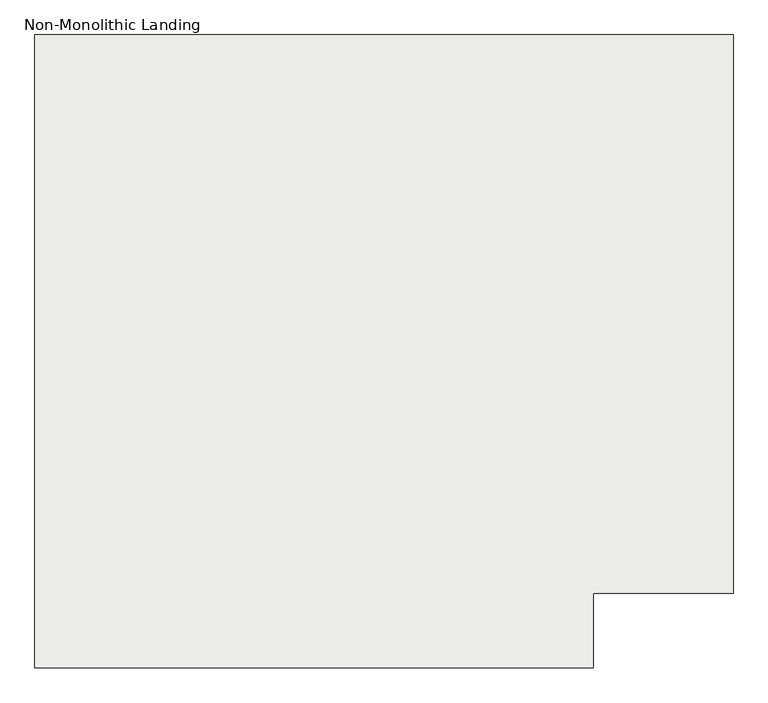
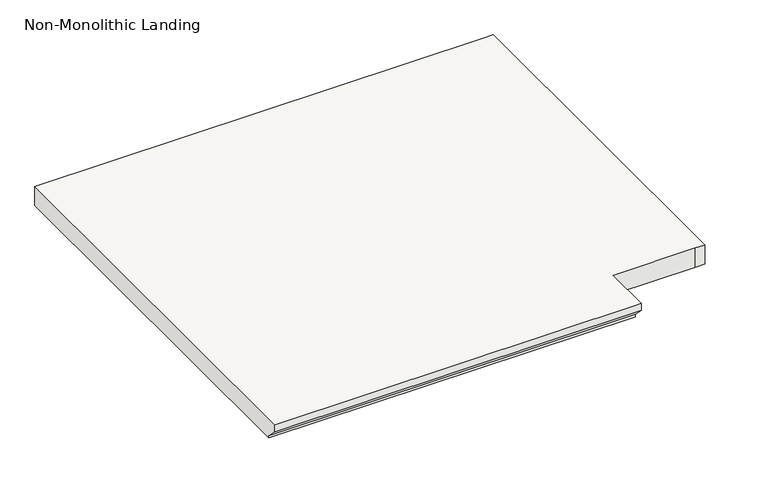
"""IFC4 building model written with IfcOpenShell, lengths in millimetres: slab geometry, Non-Monolithic Landing."""

from ifc_helpers import new_model, si_unit, origin, place, context, project, spatial, faceted_brep, source, transform, mapped, element, save


def non_monolithic_landing_e8e8d04f(model_context):
    return source(origin(), model_context, "Body", "Brep", [
        faceted_brep([(-14090.1982861, 10766.7466336, 783.0552632), (-14090.1982861, 10766.7466336, 802.1052632), (-15004.5982861, 10766.7466336, 802.1052632), (-15004.5982861, 10766.7466336, 783.0552632), (-14090.1982861, 10792.1466336, 757.6552632), (-15004.5982861, 10792.1466336, 757.6552632), (-14090.1982861, 10889.0453953, 802.1052632), (-13886.5772527, 10889.0453953, 802.1052632), (-13861.1772527, 10889.0453953, 802.1052632), (-13861.1772527, 11803.4453953, 802.1052632), (-13886.5772527, 11803.4453953, 802.1052632), (-15004.5982861, 11803.4453953, 802.1052632), (-14090.1982861, 10792.1466336, 751.3052632), (-15004.5982861, 10792.1466336, 751.3052632), (-15004.5982861, 11803.4453953, 751.3052632), (-13886.5772527, 11803.4453953, 751.3052632), (-13861.1772527, 11803.4453953, 751.3052632), (-13861.1772527, 10889.0453953, 751.3052632), (-13886.5772527, 10889.0453953, 751.3052632), (-14090.1982861, 10889.0453953, 751.3052632)], [[[0, 1, 2, 3]], [[4, 0, 3, 5]], [[6, 7, 8, 9, 10, 11, 2, 1]], [[12, 13, 14, 15, 16, 17, 18, 19]], [[13, 12, 4, 5]], [[6, 1, 0, 4, 12, 19]], [[7, 6, 19, 18]], [[8, 7, 18, 17]], [[9, 8, 17, 16]], [[10, 9, 16, 15]], [[11, 10, 15, 14]], [[2, 11, 14, 13, 5, 3]]]),
    ])


if __name__ == "__main__":
    model = new_model("IFC4")
    model_context = context("Model", 3, world=origin())
    ifc_project = project(units=[si_unit("LENGTHUNIT", "METRE", prefix="MILLI")], contexts=[model_context])
    site = spatial("IfcSite", under=ifc_project)
    building = spatial("IfcBuilding", under=site)
    placement = place(None, origin())
    non_monolithic_landing_shape = non_monolithic_landing_e8e8d04f(model_context)
    element("IfcSlab", 1, ObjectType="Non-Monolithic Landing", at=placement, inside=building, context=model_context, shape_type="MappedRepresentation", body=[
        mapped(non_monolithic_landing_shape, transform((0.0, 0.0, 0.0), x_axis=(1.0, 0.0, 0.0), y_axis=(0.0, 1.0, 0.0), z_axis=(0.0, 0.0, 1.0))),
    ])
    save(model, "model.ifc")
